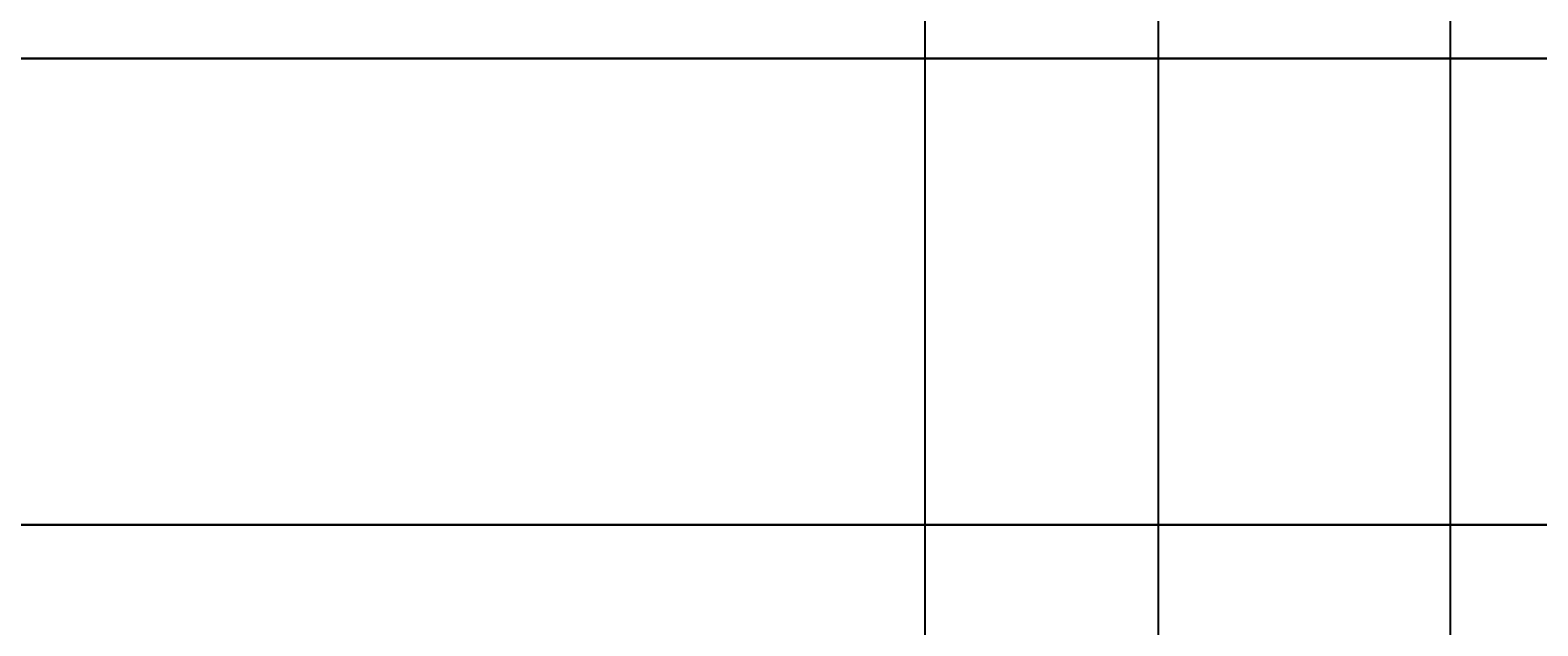
# Model space of a CAD drawing. Units: feet. Extents: x 105 to 1094, y -88 to 588.
# Tile 34 of 59: x 384 to 436, y 524 to 544. Entities that reach past the tile are written whole.
import ezdxf

# ---------------------------------------------------------------- set-up
doc = ezdxf.new("R2010")
doc.units = ezdxf.units.FT
doc.header["$MEASUREMENT"] = 0
doc.layers.add('A-ANNO-DIMS', color=2, linetype='Continuous', lineweight=18)
doc.layers.add('A-FLOR-PROJ', color=8, linetype='Continuous', lineweight=25)
doc.styles.get("Standard").update_dxf_attribs({"font": 'arial.ttf'})
doc.dimstyles.get("Standard").update_dxf_attribs({"dimtxt": 0.18, "dimasz": 0.18, "dimexe": 0.18, "dimexo": 0.0625, "dimgap": 0.09, "dimtad": 0, "dimtih": 1, "dimtoh": 1, "dimdec": 4, "dimzin": 0, "dimdsep": 46, "dimtxsty": 'Standard', "dimcen": 0.09, "dimadec": 0, "dimazin": 0, "dimtfac": 1, "dimtdec": 4, "dimtofl": 0, "dimtmove": 0, "dimatfit": 3, "dimfxl": 1, "dimtolj": 1, "dimtzin": 0, "dimarcsym": 0})

# ---------------------------------------------------------------- blocks, each defined once
blk = doc.blocks.new('*D21')
at = {"layer": 'A-ANNO-DIMS', "color": 0, "lineweight": -2, "transparency": 16777216}
for p, q in [((849.626, 543.081), (105.458, 543.081)), ((105.638, 542.901), (105.638, 250.263)), ((105.638, -42.739), (105.638, 249.899)), ((849.626, -42.919), (105.458, -42.919))]:
    blk.add_line(p, q, dxfattribs=at)
at = {"layer": 'A-ANNO-DIMS', "color": 0, "transparency": 16777216}
for points in [[(105.608, 542.901), (105.668, 542.901), (105.638, 543.081)], [(105.608, -42.739), (105.668, -42.739), (105.638, -42.919)]]:
    blk.add_solid(points, dxfattribs=at)
at = {"layer": 'Defpoints', "color": 0, "transparency": 16777216}
for p in [(105.638, 543.081), (849.688, 543.081), (849.688, -42.919)]:
    blk.add_point(p, dxfattribs=at)
at = {"layer": 'A-ANNO-DIMS', "color": 0, "transparency": 16777216, "insert": (105.638, 250.081), "char_height": 0.18, "attachment_point": 5}
blk.add_mtext('\\A1;586', dxfattribs=at)
blk = doc.blocks.new('*D24')
at = {"layer": 'A-ANNO-DIMS', "color": 0, "lineweight": -2, "transparency": 16777216}
for p, q in [((349.688, 543.144), (349.688, 588.311)), ((438.688, 527.144), (438.688, 588.311)), ((349.868, 588.131), (393.969, 588.131)), ((438.508, 588.131), (394.408, 588.131))]:
    blk.add_line(p, q, dxfattribs=at)
at = {"layer": 'A-ANNO-DIMS', "color": 0, "transparency": 16777216}
for points in [[(349.868, 588.161), (349.868, 588.101), (349.688, 588.131)], [(438.508, 588.161), (438.508, 588.101), (438.688, 588.131)]]:
    blk.add_solid(points, dxfattribs=at)
at = {"layer": 'Defpoints', "color": 0, "transparency": 16777216}
for p in [(438.688, 588.131), (349.688, 543.081), (438.688, 527.081)]:
    blk.add_point(p, dxfattribs=at)
at = {"layer": 'A-ANNO-DIMS', "color": 0, "transparency": 16777216, "insert": (394.188, 588.131), "char_height": 0.18, "attachment_point": 5}
blk.add_mtext('\\A1;89', dxfattribs=at)
blk = doc.blocks.new('*D30')
at = {"layer": 'A-ANNO-DIMS', "color": 0, "lineweight": -2, "transparency": 16777216}
for p, q in [((349.751, 543.081), (1093.918, 543.081)), ((1093.738, 542.901), (1093.738, 535.263)), ((1093.738, 527.261), (1093.738, 534.899)), ((349.751, 527.081), (1093.918, 527.081))]:
    blk.add_line(p, q, dxfattribs=at)
at = {"layer": 'A-ANNO-DIMS', "color": 0, "transparency": 16777216}
for points in [[(1093.708, 542.901), (1093.768, 542.901), (1093.738, 543.081)], [(1093.708, 527.261), (1093.768, 527.261), (1093.738, 527.081)]]:
    blk.add_solid(points, dxfattribs=at)
at = {"layer": 'Defpoints', "color": 0, "transparency": 16777216}
for p in [(349.688, 543.081), (349.688, 527.081), (1093.738, 527.081)]:
    blk.add_point(p, dxfattribs=at)
at = {"layer": 'A-ANNO-DIMS', "color": 0, "transparency": 16777216, "insert": (1093.738, 535.081), "char_height": 0.18, "attachment_point": 5}
blk.add_mtext('\\A1;16', dxfattribs=at)
blk = doc.blocks.new('*D52')
at = {"layer": 'A-ANNO-DIMS', "color": 0, "lineweight": -2, "transparency": 16777216}
for p, q in [((414.688, 394.144), (414.688, 588.311)), ((432.688, 394.144), (432.688, 588.311)), ((414.868, 588.131), (423.478, 588.131)), ((432.508, 588.131), (423.899, 588.131))]:
    blk.add_line(p, q, dxfattribs=at)
at = {"layer": 'A-ANNO-DIMS', "color": 0, "transparency": 16777216}
for points in [[(414.868, 588.161), (414.868, 588.101), (414.688, 588.131)], [(432.508, 588.161), (432.508, 588.101), (432.688, 588.131)]]:
    blk.add_solid(points, dxfattribs=at)
at = {"layer": 'Defpoints', "color": 0, "transparency": 16777216}
for p in [(414.688, 588.131), (414.688, 394.081), (432.688, 394.081)]:
    blk.add_point(p, dxfattribs=at)
at = {"layer": 'A-ANNO-DIMS', "color": 0, "transparency": 16777216, "insert": (423.688, 588.131), "char_height": 0.18, "attachment_point": 5}
blk.add_mtext('\\A1;18', dxfattribs=at)
blk = doc.blocks.new('*D53')
at = {"layer": 'A-ANNO-DIMS', "color": 0, "lineweight": -2, "transparency": 16777216}
for p, q in [((365.688, 394.144), (365.688, 588.311)), ((414.688, 394.144), (414.688, 588.311)), ((365.868, 588.131), (389.966, 588.131)), ((414.508, 588.131), (390.411, 588.131))]:
    blk.add_line(p, q, dxfattribs=at)
at = {"layer": 'A-ANNO-DIMS', "color": 0, "transparency": 16777216}
for points in [[(365.868, 588.161), (365.868, 588.101), (365.688, 588.131)], [(414.508, 588.161), (414.508, 588.101), (414.688, 588.131)]]:
    blk.add_solid(points, dxfattribs=at)
at = {"layer": 'Defpoints', "color": 0, "transparency": 16777216}
for p in [(365.688, 588.131), (365.688, 394.081), (414.688, 394.081)]:
    blk.add_point(p, dxfattribs=at)
at = {"layer": 'A-ANNO-DIMS', "color": 0, "transparency": 16777216, "insert": (390.188, 588.131), "char_height": 0.18, "attachment_point": 5}
blk.add_mtext('\\A1;49', dxfattribs=at)
blk = doc.blocks.new('*D56')
at = {"layer": 'A-ANNO-DIMS', "color": 0, "lineweight": -2, "transparency": 16777216}
for p, q in [((374.688, 252.144), (374.688, 588.311)), ((422.688, 252.144), (422.688, 588.311)), ((374.868, 588.131), (398.466, 588.131)), ((422.508, 588.131), (398.911, 588.131))]:
    blk.add_line(p, q, dxfattribs=at)
at = {"layer": 'A-ANNO-DIMS', "color": 0, "transparency": 16777216}
for points in [[(374.868, 588.161), (374.868, 588.101), (374.688, 588.131)], [(422.508, 588.161), (422.508, 588.101), (422.688, 588.131)]]:
    blk.add_solid(points, dxfattribs=at)
at = {"layer": 'Defpoints', "color": 0, "transparency": 16777216}
for p in [(422.688, 588.131), (374.688, 252.081), (422.688, 252.081)]:
    blk.add_point(p, dxfattribs=at)
at = {"layer": 'A-ANNO-DIMS', "color": 0, "transparency": 16777216, "insert": (398.688, 588.131), "char_height": 0.18, "attachment_point": 5}
blk.add_mtext('\\A1;48', dxfattribs=at)

msp = doc.modelspace()

# ---------------------------------------------------------------- linework, layer by layer
at = {"layer": 'A-FLOR-PROJ'}
msp.add_line((438.6883, 527.0812), (349.6883, 527.0812), dxfattribs=at)

# ---------------------------------------------------------------- dimensions: what is measured, and where the dimension line sits
at = {"layer": 'A-ANNO-DIMS'}
for base, p1, p2, picture, middle in [((438.6883, 588.1312), (349.6883, 543.0812), (438.6883, 527.0812), '*D24', (394.1883, 588.1312)), ((365.6883, 588.1312), (414.6883, 394.0812), (365.6883, 394.0812), '*D53', (390.1883, 588.1312)), ((422.6883, 588.1312), (374.6883, 252.0812), (422.6883, 252.0812), '*D56', (398.6883, 588.1312)), ((414.6883, 588.1312), (432.6883, 394.0812), (414.6883, 394.0812), '*D52', (423.6883, 588.1312))]:
    dim = msp.add_linear_dim(base=base, p1=p1, p2=p2, dimstyle='Standard', override={"dimdec": 0, "dimlfac": 1, "dimrnd": 0, "dimzin": 0, "dimdsep": 46, "dimlunit": 2}, dxfattribs=at)
    dim.commit()
    dim.dimension.update_dxf_attribs({"geometry": picture, "text_midpoint": middle})
for base, p1, p2, picture, middle in [((105.6383, 543.0812), (849.6883, -42.9188), (849.6883, 543.0812), '*D21', (105.6383, 250.0812)), ((1093.7383, 527.0812), (349.6883, 543.0812), (349.6883, 527.0812), '*D30', (1093.7383, 535.0812))]:
    dim = msp.add_linear_dim(base=base, p1=p1, p2=p2, angle=90, dimstyle='Standard', override={"dimdec": 0, "dimlfac": 1, "dimrnd": 0, "dimzin": 0, "dimdsep": 46, "dimlunit": 2}, dxfattribs=at)
    dim.commit()
    dim.dimension.update_dxf_attribs({"geometry": picture, "text_midpoint": middle})

doc.saveas('drawing.dxf')
